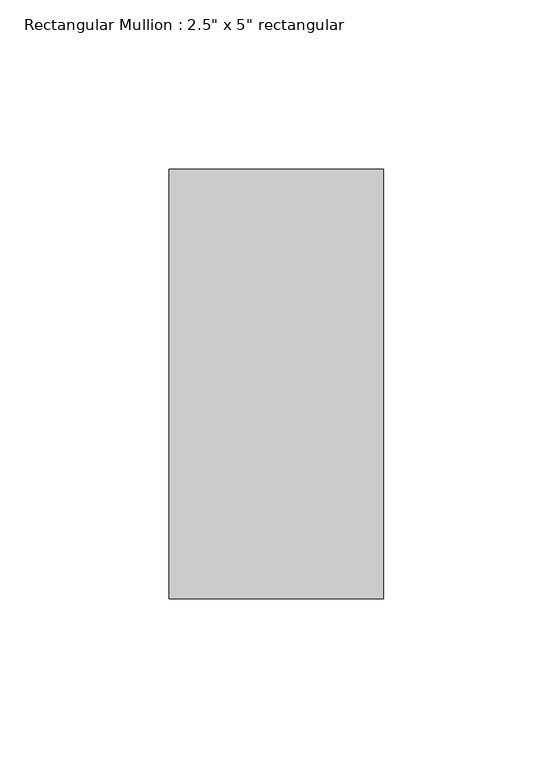
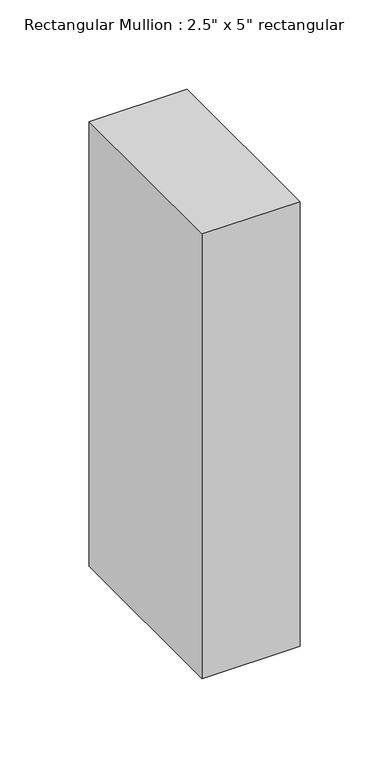
"""IFC4 building model written with IfcOpenShell, lengths in millimetres: member geometry."""

from ifc_helpers import new_model, si_unit, frame, origin, place, context, project, spatial, polyline, outline, extrude, source, transform, mapped, element, save


def member_3c3dc66a(model_context):
    return source(origin(), model_context, "Body", "SweptSolid", [
        extrude(outline(polyline([(0.0, 63.5), (0.0, -63.5), (-63.5, -63.5), (-63.5, 63.5), (0.0, 63.5)])), frame((0.0, 0.0, -304.8), z_axis=(0.0, 0.0, 1.0), x_axis=(1.0, 0.0, 0.0)), (0.0, 0.0, 1.0), 304.8),
    ])


if __name__ == "__main__":
    model = new_model("IFC4")
    model_context = context("Model", 3, world=origin())
    ifc_project = project(units=[si_unit("LENGTHUNIT", "METRE", prefix="MILLI")], contexts=[model_context])
    site = spatial("IfcSite", under=ifc_project)
    building = spatial("IfcBuilding", under=site)
    placement = place(None, origin())
    member_shape = member_3c3dc66a(model_context)
    element("IfcMember", 1, ObjectType="Rectangular Mullion : 2.5\" x 5\" rectangular", at=placement, inside=building, context=model_context, shape_type="MappedRepresentation", body=[
        mapped(member_shape, transform((0.0, 0.0, 0.0), x_axis=(1.0, 0.0, 0.0), y_axis=(0.0, 1.0, 0.0), z_axis=(0.0, 0.0, 1.0))),
    ])
    save(model, "model.ifc")

# Revit data of these elements
# Type "Rectangular Mullion : 2.5\" x 5\" rectangular"
#   built-in parameter 1007304 = 0.416667 (stored number, unit not read)
#   built-in parameter 1007301 = 0.104167 (stored number, unit not read)
#   built-in parameter 1007300 = 0.104167 (stored number, unit not read)
# Element 1 (IfcMember, "Rectangular Mullion : 2.5\" x 5\" rectangular")
#   Materials on its faces: "door colour"
# Materials
#   "door colour": class "Generic", colour RGB 120 120 120, transparency 0, Cost = 0
